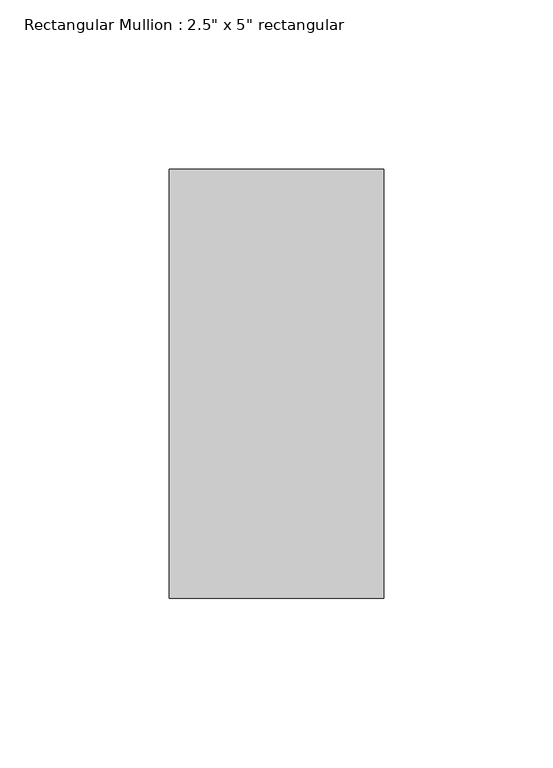
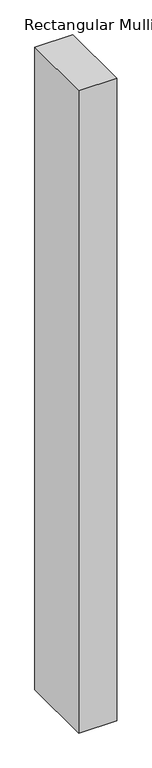
"""IFC4 building model written with IfcOpenShell, lengths in millimetres: member geometry."""

from ifc_helpers import new_model, si_unit, frame, origin, place, context, project, spatial, polyline, outline, extrude, source, transform, mapped, element, save


def member_a8685e1c(model_context):
    return source(origin(), model_context, "Body", "SweptSolid", [
        extrude(outline(polyline([(0.0, 63.5), (0.0, -63.5), (-63.5, -63.5), (-63.5, 63.5), (0.0, 63.5)])), frame((0.0, 0.0, -1136.6499998), z_axis=(0.0, 0.0, 1.0), x_axis=(1.0, 0.0, 0.0)), (0.0, 0.0, 1.0), 1136.6499998),
    ])


if __name__ == "__main__":
    model = new_model("IFC4")
    model_context = context("Model", 3, world=origin())
    ifc_project = project(units=[si_unit("LENGTHUNIT", "METRE", prefix="MILLI")], contexts=[model_context])
    site = spatial("IfcSite", under=ifc_project)
    building = spatial("IfcBuilding", under=site)
    placement = place(None, origin())
    member_shape = member_a8685e1c(model_context)
    element("IfcMember", 1, ObjectType="Rectangular Mullion : 2.5\" x 5\" rectangular", at=placement, inside=building, context=model_context, shape_type="MappedRepresentation", body=[
        mapped(member_shape, transform((0.0, 0.0, 0.0), x_axis=(1.0, 0.0, 0.0), y_axis=(0.0, 1.0, 0.0), z_axis=(0.0, 0.0, 1.0))),
    ])
    save(model, "model.ifc")

# Revit data of these elements
# Type "Rectangular Mullion : 2.5\" x 5\" rectangular"
#   built-in parameter 1007304 = 0.416667 (stored number, unit not read)
#   built-in parameter 1007301 = 0.104167 (stored number, unit not read)
#   built-in parameter 1007300 = 0.104167 (stored number, unit not read)
# Element 1 (IfcMember, "Rectangular Mullion : 2.5\" x 5\" rectangular")
#   Materials on its faces: "BLACK COLOUR"
# Materials
#   "BLACK COLOUR": class "Generic", colour RGB 120 120 120, transparency 0, Cost = 0
